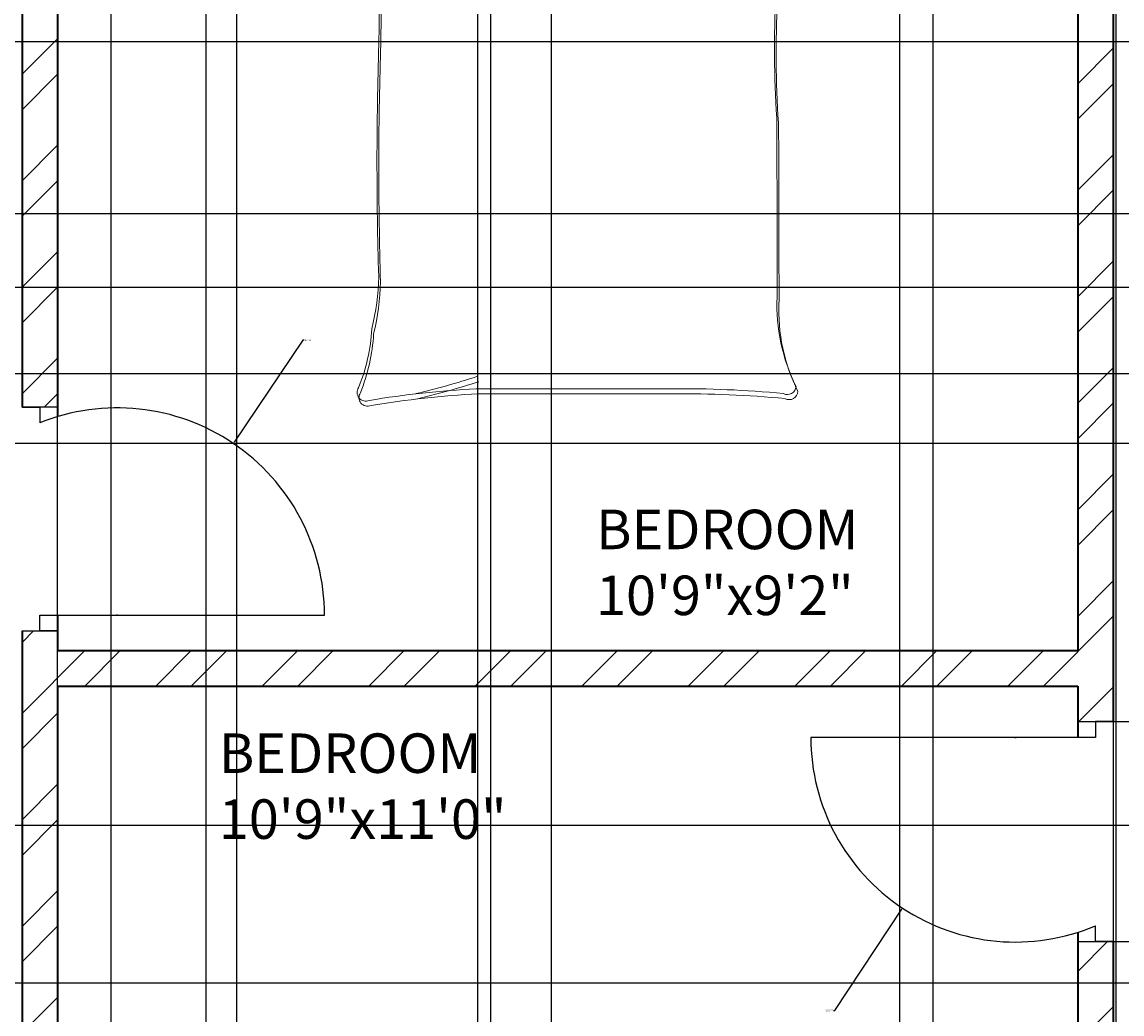
# Model space of a CAD drawing. Units: inches. Extents: x 2529 to 3014, y 1203 to 2262.
# Tile 11 of 13: x 2733 to 2872, y 2008 to 2133. Entities that reach past the tile are written whole.
import ezdxf

# ---------------------------------------------------------------- set-up
doc = ezdxf.new("R2010")
doc.units = ezdxf.units.IN
for name, color, linetype, lineweight in [('A-ANNO-DIMS', 2, 'Continuous', 18), ('A-AREA-IDEN', 7, 'Continuous', 18), ('A-DOOR', 21, 'Continuous', 25), ('A-FURN', 8, 'Continuous', 18), ('A-WALL', 7, 'Continuous', 35), ('A-WALL-PATT', 143, 'Continuous', 13)]:
    doc.layers.add(name, color=color, linetype=linetype, lineweight=lineweight)
doc.styles.get("Standard").update_dxf_attribs({"font": 'arial.ttf'})
doc.dimstyles.get("Standard").update_dxf_attribs({"dimtxt": 0.18, "dimasz": 0.18, "dimexe": 0.18, "dimexo": 0.0625, "dimgap": 0.09, "dimtad": 0, "dimtih": 1, "dimtoh": 1, "dimdec": 4, "dimzin": 0, "dimdsep": 46, "dimtxsty": 'Standard', "dimcen": 0.09, "dimadec": 0, "dimazin": 0, "dimtfac": 1, "dimtdec": 4, "dimtofl": 0, "dimtmove": 0, "dimatfit": 3, "dimfxl": 1, "dimtolj": 1, "dimtzin": 0, "dimarcsym": 0})

# ---------------------------------------------------------------- blocks, each defined once
blk = doc.blocks.new('BED-DOUBLE')
for p, q in [((3.48, 63.33), (3.48, 81.44)), ((3.48, 63.33), (3.48, 81.44)), ((3.48, 81.44), (51.49, 81.44)), ((3.7, 62.69), (3.7, 80.8)), ((3.7, 62.69), (3.7, 80.8)), ((51.27, 81.44), (51.27, 54.83)), ((51.27, 81.44), (51.27, 54.83)), ((51.49, 81.44), (51.49, 80.8)), ((51.49, 80.8), (51.49, 54.19)), ((51.49, 80.8), (51.49, 54.19)), ((3.48, 79.91), (51.27, 79.91)), ((3.48, 79.91), (51.27, 79.91)), ((24.54, 78.99), (25.98, 79.57)), ((24.54, 78.99), (25.98, 79.57)), ((25.98, 79.57), (26.56, 74.22)), ((25.98, 79.57), (26.56, 74.22)), ((3.7, 79.27), (51.49, 79.27)), ((3.7, 79.27), (51.49, 79.27)), ((3.9, 78.11), (8.18, 78.43)), ((3.9, 78.11), (8.18, 78.43)), ((3.9, 78.13), (4.47, 74.95)), ((3.9, 78.13), (4.47, 74.95)), ((8.18, 78.43), (8.29, 78.42)), ((8.18, 78.43), (8.29, 78.42)), ((8.29, 78.42), (12.11, 78.13)), ((8.29, 78.42), (12.11, 78.13)), ((12.11, 78.13), (17.6, 77.12)), ((12.11, 78.13), (17.6, 77.12)), ((14.86, 77.69), (16.88, 78.42)), ((14.86, 77.69), (16.88, 78.42)), ((16.88, 78.42), (19.77, 79.14)), ((16.88, 78.42), (19.77, 79.14)), ((17.11, 77.78), (20, 78.5)), ((17.11, 77.78), (20, 78.5)), ((19.77, 79.14), (20.09, 79.14)), ((19.77, 79.14), (20.09, 79.14)), ((20, 78.5), (20.32, 78.5)), ((20, 78.5), (20.32, 78.5)), ((20.09, 79.14), (24.54, 78.99)), ((20.09, 79.14), (24.54, 78.99)), ((20.32, 78.5), (24.77, 78.36)), ((20.32, 78.5), (24.77, 78.36)), ((24.77, 78.36), (26.21, 78.93)), ((24.77, 78.36), (26.21, 78.93)), ((26.21, 78.93), (26.79, 73.58)), ((26.21, 78.93), (26.79, 73.58)), ((27.98, 78.95), (27.73, 73.58)), ((27.98, 78.95), (27.73, 73.58)), ((28.21, 78.31), (27.96, 72.94)), ((28.21, 78.31), (27.96, 72.94)), ((29.46, 78.46), (27.98, 78.95)), ((29.46, 78.46), (27.98, 78.95)), ((29.68, 77.83), (28.21, 78.31)), ((29.68, 77.83), (28.21, 78.31)), ((33.88, 78.89), (29.46, 78.46)), ((33.88, 78.89), (29.46, 78.46)), ((34.11, 78.25), (29.68, 77.83)), ((34.11, 78.25), (29.68, 77.83)), ((34.21, 78.91), (33.88, 78.89)), ((34.21, 78.91), (33.88, 78.89)), ((34.43, 78.27), (34.11, 78.25)), ((34.43, 78.27), (34.11, 78.25)), ((37.14, 78.37), (34.21, 78.91)), ((37.14, 78.37), (34.21, 78.91)), ((37.36, 77.73), (34.43, 78.27)), ((37.36, 77.73), (34.43, 78.27)), ((41.91, 78.37), (36.5, 77.02)), ((41.91, 78.37), (36.5, 77.02)), ((39.2, 77.77), (37.14, 78.37)), ((39.2, 77.77), (37.14, 78.37)), ((45.71, 78.9), (41.91, 78.37)), ((45.71, 78.9), (41.91, 78.37)), ((45.94, 78.26), (42.14, 77.73)), ((45.94, 78.26), (42.14, 77.73)), ((50.11, 78.89), (44.71, 78.98)), ((44.71, 78.98), (45.71, 78.9)), ((50.11, 78.89), (44.71, 78.98)), ((44.71, 78.98), (45.71, 78.9)), ((50.34, 78.25), (44.94, 78.34)), ((44.94, 78.34), (45.94, 78.26)), ((50.34, 78.25), (44.94, 78.34)), ((44.94, 78.34), (45.94, 78.26)), ((50.11, 78.89), (49.73, 75.68)), ((50.11, 78.89), (49.73, 75.68)), ((50.34, 78.25), (49.96, 75.04)), ((50.34, 78.25), (49.96, 75.04)), ((4.12, 77.49), (4.7, 74.31)), ((4.12, 77.49), (4.7, 74.31)), ((4.13, 77.47), (8.41, 77.8)), ((4.13, 77.47), (8.41, 77.8)), ((8.41, 77.8), (8.51, 77.78)), ((8.41, 77.8), (8.51, 77.78)), ((8.51, 77.78), (12.34, 77.49)), ((8.51, 77.78), (12.34, 77.49)), ((12.34, 77.49), (17.83, 76.48)), ((12.34, 77.49), (17.83, 76.48)), ((15.08, 77.05), (17.11, 77.78)), ((15.08, 77.05), (17.11, 77.78)), ((42.14, 77.73), (36.72, 76.38)), ((42.14, 77.73), (36.72, 76.38)), ((39.43, 77.13), (37.36, 77.73)), ((39.43, 77.13), (37.36, 77.73)), ((5.05, 72.49), (6.06, 75.24)), ((5.05, 72.49), (6.06, 75.24)), ((49.31, 73.19), (48.13, 75.87)), ((49.31, 73.19), (48.13, 75.87)), ((49.54, 72.55), (48.36, 75.23)), ((49.54, 72.55), (48.36, 75.23)), ((49.73, 75.68), (50.33, 73.11)), ((49.73, 75.68), (50.33, 73.11)), ((4.47, 74.95), (4.04, 72.34)), ((4.47, 74.95), (4.04, 72.34)), ((4.7, 74.31), (4.27, 71.7)), ((4.7, 74.31), (4.27, 71.7)), ((5.28, 71.85), (6.29, 74.6)), ((5.28, 71.85), (6.29, 74.6)), ((26.56, 74.22), (27.14, 71.04)), ((26.56, 74.22), (27.14, 71.04)), ((49.96, 75.04), (50.56, 72.47)), ((49.96, 75.04), (50.56, 72.47)), ((4.04, 72.34), (4.62, 71.33)), ((4.04, 72.34), (4.62, 71.33)), ((4.47, 68.87), (5.05, 72.49)), ((4.47, 68.87), (5.05, 72.49)), ((26.79, 73.58), (27.37, 70.4)), ((26.79, 73.58), (27.37, 70.4)), ((27.73, 73.58), (27.36, 70.37)), ((27.73, 73.58), (27.36, 70.37)), ((27.96, 72.94), (27.58, 69.73)), ((27.96, 72.94), (27.58, 69.73)), ((50.11, 69.61), (49.31, 73.19)), ((50.11, 69.61), (49.31, 73.19)), ((50.34, 68.98), (49.54, 72.55)), ((50.34, 68.98), (49.54, 72.55)), ((50.33, 73.11), (49.81, 72.06)), ((50.33, 73.11), (49.82, 72.06)), ((50.56, 72.47), (50.04, 71.42)), ((50.56, 72.47), (50.04, 71.42)), ((4.27, 71.7), (4.85, 70.69)), ((4.27, 71.7), (4.85, 70.69)), ((4.7, 68.23), (5.28, 71.85)), ((4.7, 68.23), (5.28, 71.85)), ((27.14, 71.04), (27.14, 69.74)), ((27.14, 71.04), (27.14, 69.74)), ((27.14, 69.74), (26.56, 67.86)), ((27.14, 69.74), (26.56, 67.86)), ((27.36, 70.37), (27.44, 69.07)), ((27.36, 70.37), (27.44, 69.07)), ((27.37, 70.4), (27.37, 69.1)), ((27.37, 70.4), (27.37, 69.1)), ((27.58, 69.73), (27.67, 68.43)), ((27.58, 69.73), (27.66, 68.43)), ((49.92, 68.01), (50.11, 69.61)), ((49.92, 68.01), (50.11, 69.61)), ((4.76, 67.28), (4.47, 68.87)), ((4.76, 67.28), (4.47, 68.87)), ((4.99, 66.64), (4.7, 68.23)), ((4.99, 66.64), (4.7, 68.23)), ((27.37, 69.1), (26.79, 67.22)), ((27.37, 69.1), (26.79, 67.22)), ((27.44, 69.07), (28.13, 67.23)), ((27.44, 69.07), (28.13, 67.23)), ((27.66, 68.43), (28.36, 66.59)), ((27.67, 68.43), (28.36, 66.59)), ((50.15, 67.37), (50.34, 68.98)), ((50.15, 67.37), (50.34, 68.98)), ((4.18, 64.1), (4.76, 67.28)), ((4.18, 64.1), (4.76, 67.28)), ((26.56, 67.86), (26.56, 65.18)), ((26.56, 67.86), (26.56, 65.18)), ((26.79, 67.22), (26.79, 64.54)), ((26.79, 67.22), (26.79, 64.54)), ((28.13, 67.23), (28.3, 64.55)), ((28.13, 67.23), (28.3, 64.55)), ((50.7, 64.87), (49.92, 68.01)), ((50.7, 64.87), (49.92, 68.01)), ((50.93, 64.23), (50.15, 67.37)), ((50.93, 64.23), (50.15, 67.37)), ((4.41, 63.46), (4.99, 66.64)), ((4.41, 63.46), (4.99, 66.64)), ((6.38, 65.81), (10.41, 65.15)), ((6.38, 65.81), (10.41, 65.15)), ((24.1, 65.18), (20.96, 66.27)), ((24.1, 65.18), (20.96, 66.27)), ((24.33, 64.54), (21.19, 65.63)), ((24.33, 64.54), (21.19, 65.63)), ((28.36, 66.59), (28.53, 63.91)), ((28.36, 66.59), (28.53, 63.91)), ((30.75, 64.7), (33.82, 65.99)), ((30.75, 64.7), (33.82, 65.99)), ((32.56, 65.81), (36.6, 65.15)), ((32.56, 65.81), (36.6, 65.15)), ((9.28, 64.83), (4.18, 64.1)), ((9.28, 64.83), (4.18, 64.1)), ((9.51, 64.19), (4.41, 63.46)), ((9.51, 64.19), (4.41, 63.46)), ((6.61, 65.18), (10.64, 64.51)), ((6.61, 65.18), (10.64, 64.51)), ((10.41, 65.15), (9.28, 64.83)), ((10.41, 65.15), (9.28, 64.83)), ((10.64, 64.51), (9.51, 64.19)), ((10.64, 64.51), (9.51, 64.19)), ((10.41, 65.15), (17.42, 64.72)), ((10.41, 65.15), (17.42, 64.72)), ((10.64, 64.51), (17.65, 64.08)), ((10.64, 64.51), (17.65, 64.08)), ((17.42, 64.72), (19.38, 65.27)), ((17.42, 64.72), (19.38, 65.27)), ((17.65, 64.08), (19.61, 64.64)), ((17.65, 64.08), (19.61, 64.64)), ((19.38, 65.27), (24.52, 64.87)), ((19.38, 65.27), (24.52, 64.87)), ((19.61, 64.64), (24.74, 64.23)), ((19.61, 64.64), (24.74, 64.23)), ((26.56, 65.18), (24.1, 65.18)), ((26.56, 65.18), (24.1, 65.18)), ((26.79, 64.54), (24.33, 64.54)), ((26.79, 64.54), (24.33, 64.54)), ((28.3, 64.55), (30.75, 64.7)), ((28.3, 64.55), (30.75, 64.7)), ((28.53, 63.91), (30.98, 64.06)), ((28.53, 63.91), (30.98, 64.06)), ((30.26, 64.06), (34.45, 57.57)), ((30.26, 64.06), (34.45, 57.57)), ((30.98, 64.06), (34.05, 65.35)), ((30.98, 64.06), (34.05, 65.35)), ((40.64, 61.13), (32.31, 64.06)), ((40.64, 61.13), (32.31, 64.06)), ((32.79, 65.18), (36.83, 64.51)), ((32.79, 65.18), (36.82, 64.51)), ((36.6, 65.15), (43.61, 64.72)), ((36.6, 65.15), (43.61, 64.72)), ((36.82, 64.51), (43.83, 64.08)), ((36.83, 64.51), (43.84, 64.08)), ((43.61, 64.72), (45.57, 65.27)), ((43.61, 64.72), (45.57, 65.27)), ((43.83, 64.08), (45.8, 64.64)), ((43.84, 64.08), (45.8, 64.64)), ((45.57, 65.27), (50.7, 64.87)), ((45.57, 65.27), (50.7, 64.87)), ((45.8, 64.64), (50.93, 64.23)), ((45.8, 64.64), (50.93, 64.23)), ((30.49, 63.42), (34.68, 56.93)), ((30.49, 63.42), (34.68, 56.93)), ((40.87, 60.49), (32.53, 63.42)), ((40.87, 60.49), (32.54, 63.42)), ((46.22, 59.11), (40.64, 61.13)), ((46.22, 59.11), (40.64, 61.13)), ((46.45, 58.48), (40.87, 60.49)), ((46.45, 58.48), (40.87, 60.49)), ((49.16, 56.95), (46.22, 59.11)), ((49.16, 56.95), (46.22, 59.11)), ((49.39, 56.31), (46.45, 58.48)), ((49.39, 56.31), (46.45, 58.48)), ((34.45, 57.57), (36.15, 53.08)), ((34.45, 57.57), (36.15, 53.08)), ((34.68, 56.93), (36.38, 52.44)), ((34.68, 56.93), (36.38, 52.44)), ((52.87, 53.7), (49.16, 56.95)), ((52.87, 53.7), (49.16, 56.95)), ((53.1, 53.06), (49.39, 56.31)), ((53.1, 53.06), (49.39, 56.31)), ((36.15, 53.08), (36.46, 51.07)), ((36.15, 53.08), (36.46, 51.07)), ((40.95, 52.61), (44.36, 53.08)), ((40.95, 52.61), (44.36, 53.08)), ((44.36, 53.08), (48.23, 53.39)), ((44.36, 53.08), (48.23, 53.39)), ((48.23, 53.39), (51.33, 53.08)), ((48.23, 53.39), (51.33, 53.08)), ((51.33, 53.08), (52.87, 53.7)), ((51.33, 53.08), (52.87, 53.7)), ((51.56, 52.44), (53.1, 53.06)), ((51.56, 52.44), (53.1, 53.06)), ((52.95, 51.95), (52.87, 53.7, 3.87)), ((52.95, 51.95), (52.87, 53.7, 3.87)), ((53.18, 51.31), (53.1, 53.06, 3.87)), ((53.18, 51.31), (53.1, 53.06, 3.87)), ((36.38, 52.44), (36.69, 50.43)), ((36.38, 52.44), (36.69, 50.43)), ((36.46, 51.07), (38.94, 51.69)), ((36.46, 51.07), (38.94, 51.69)), ((38.94, 51.69), (40.95, 52.61)), ((38.94, 51.69), (40.95, 52.61)), ((39.17, 51.05), (41.18, 51.97)), ((39.17, 51.05), (41.18, 51.97)), ((41.18, 51.97), (44.59, 52.44)), ((41.18, 51.97), (44.59, 52.44)), ((44.59, 52.44), (48.46, 52.75)), ((44.59, 52.44), (48.46, 52.75)), ((48.46, 52.75), (51.56, 52.44)), ((48.46, 52.75), (51.56, 52.44)), ((36.69, 50.43), (39.17, 51.05)), ((36.69, 50.43), (39.17, 51.05)), ((15.06, 2.2), (39.68, 2.2)), ((15.06, 2.2), (39.68, 2.2)), ((15.29, 1.56), (39.91, 1.56)), ((15.29, 1.56), (39.91, 1.56))]:
    blk.add_line(p, q)
for centre, radius, start, end in [((21.36, -100.61), 164.97, 86.0865, 96.7821), ((21.36, -100.61), 164.97, 86.0865, 96.7821), ((85.16, 61.35), 83.31, 178.7218, 185.604), ((85.16, 61.35), 83.31, 178.7218, 185.604), ((21.59, -101.25), 164.97, 86.0865, 96.7821), ((21.59, -101.25), 164.97, 86.0865, 96.7821), ((85.39, 60.71), 83.31, 178.7218, 185.604), ((85.39, 60.71), 83.31, 178.7218, 185.604), ((17.76, -74.87), 129.02, 81.7845, 96.9006), ((17.76, -74.87), 129.02, 81.7845, 96.9006), ((17.98, -75.51), 129.02, 81.7845, 96.9006), ((17.98, -75.51), 129.02, 81.7845, 96.9006), ((-167.31, 50.27), 170.11, 358.4762, 1.0082), ((-167.31, 50.27), 170.11, 358.4762, 1.0082), ((-167.08, 49.63), 170.11, 358.4762, 1.0082), ((-167.08, 49.63), 170.11, 358.4762, 1.0082), ((31.15, 79.96), 29.65, 280.6617, 289.8806), ((31.15, 79.96), 29.65, 280.6617, 289.8806), ((43.74, 46.38), 6.22, 78.6608, 113.7384), ((43.74, 46.38), 6.22, 78.6608, 113.7384), ((43.97, 45.74), 6.22, 78.6608, 113.7384), ((43.97, 45.74), 6.22, 78.6608, 113.7384), ((51.33, 88.1), 36.18, 259.8763, 272.5657), ((51.33, 88.1), 36.18, 259.8763, 272.5657), ((51.56, 87.46), 36.18, 259.8763, 272.5657), ((51.56, 87.46), 36.18, 259.8763, 272.5657), ((182.27, 45.13), 129.5, 176.9791, 183.8365), ((182.27, 45.13), 129.5, 176.9791, 183.8365), ((36.64, 51), 0.185, 160.2464, 271.1377), ((36.64, 51), 0.185, 160.2464, 271.1377), ((36.87, 50.36), 0.185, 160.2464, 271.1377), ((36.86, 50.36), 0.185, 160.2464, 271.1377), ((31.38, 79.32), 29.65, 280.6617, 289.8806), ((31.38, 79.32), 29.65, 280.6617, 289.8806), ((182.49, 44.49), 129.5, 176.9791, 183.8365), ((182.49, 44.49), 129.5, 176.9791, 183.8365), ((484.82, 30.83), 482.31, 178.2277, 181.7185), ((484.82, 30.83), 482.31, 178.2277, 181.7185), ((485.05, 30.19), 482.31, 178.2277, 181.7185), ((485.05, 30.19), 482.31, 178.2277, 181.7185), ((-4508.74, 13.62), 4561.86, 0.00217, 0.28689), ((-4508.74, 13.62), 4561.86, 0.00217, 0.28689), ((-4508.51, 12.98), 4561.86, 0.00217, 0.28689), ((-4508.51, 12.98), 4561.86, 0.00217, 0.28689), ((-26.9, 16.93), 29.63, 346.0648, 358.9113), ((-26.9, 16.93), 29.63, 346.0648, 358.9113), ((-26.67, 16.29), 29.63, 346.0648, 358.9113), ((-26.67, 16.29), 29.63, 346.0648, 358.9113), ((76.16, 12.78), 23.07, 177.4714, 206.4681), ((76.16, 12.78), 23.07, 177.4714, 206.4681), ((76.39, 12.14), 23.07, 177.4714, 206.4681), ((76.39, 12.14), 23.07, 177.4714, 206.4681), ((-21.66, 11.17), 23.56, 337.9751, 356.652), ((-21.66, 11.17), 23.56, 337.9751, 356.652), ((-21.43, 10.53), 23.56, 337.9751, 356.652), ((-21.43, 10.53), 23.56, 337.9751, 356.652), ((-17.22, 105.16), 106.46, 283.3832, 287.7053), ((-17.22, 105.16), 106.46, 283.3832, 287.7053), ((-16.99, 104.52), 106.46, 283.3832, 287.7053), ((-16.99, 104.52), 106.46, 283.3832, 287.7053), ((1.09, 1.73), 1.09, 146.1736, 293.4781), ((1.09, 1.73), 1.09, 146.1736, 293.4781), ((1.32, 1.09), 1.09, 146.1736, 293.4781), ((1.32, 1.09), 1.09, 146.1736, 293.4781), ((21.43, -119.39), 121.76, 92.9958, 99.4091), ((21.43, -119.39), 121.76, 92.9958, 99.4091), ((21.66, -120.03), 121.76, 92.9958, 99.4091), ((21.66, -120.03), 121.76, 92.9958, 99.4091), ((41.15, -130.83), 133.04, 84.4998, 90.6351), ((41.15, -130.83), 133.04, 84.4998, 90.6351), ((41.38, -131.47), 133.04, 84.4998, 90.6351), ((41.38, -131.47), 133.04, 84.4998, 90.6351), ((54.41, 2.57), 1.1, 242.6588, 356.02), ((54.41, 2.57), 1.1, 242.6588, 356.02), ((54.64, 1.93), 1.1, 242.6588, 356.02), ((54.64, 1.93), 1.1, 242.6588, 356.02)]:
    blk.add_arc(centre, radius, start, end)
blk = doc.blocks.new('*D36')
at = {"layer": 'A-ANNO-DIMS', "color": 0, "lineweight": -2, "transparency": 16777216}
for p, q in [((2737.56, 1582.57), (2737.56, 2243.11)), ((2737.74, 2242.93), (2746.49, 2242.93)), ((2756.15, 2242.93), (2747.4, 2242.93)), ((2756.33, 1582.57), (2756.33, 2243.11))]:
    blk.add_line(p, q, dxfattribs=at)
at = {"layer": 'A-ANNO-DIMS', "color": 0, "transparency": 16777216}
for points in [[(2737.74, 2242.96), (2737.74, 2242.9), (2737.56, 2242.93)], [(2756.15, 2242.96), (2756.15, 2242.9), (2756.33, 2242.93)]]:
    blk.add_solid(points, dxfattribs=at)
at = {"layer": 'Defpoints', "color": 0, "transparency": 16777216}
for p in [(2756.33, 2242.93), (2737.56, 1582.5), (2756.33, 1582.5)]:
    blk.add_point(p, dxfattribs=at)
at = {"layer": 'A-ANNO-DIMS', "color": 0, "transparency": 16777216, "insert": (2746.94, 2242.93), "char_height": 0.18, "attachment_point": 5}
blk.add_mtext('\\A1;18.778', dxfattribs=at)
blk = doc.blocks.new('*D37')
at = {"layer": 'A-ANNO-DIMS', "color": 0, "lineweight": -2, "transparency": 16777216}
for p, q in [((2756.33, 1582.57), (2756.33, 2243.11)), ((2756.51, 2242.93), (2774.11, 2242.93)), ((2792.15, 2242.93), (2774.55, 2242.93)), ((2792.33, 1582.57), (2792.33, 2243.11))]:
    blk.add_line(p, q, dxfattribs=at)
at = {"layer": 'A-ANNO-DIMS', "color": 0, "transparency": 16777216}
for points in [[(2756.51, 2242.96), (2756.51, 2242.9), (2756.33, 2242.93)], [(2792.15, 2242.96), (2792.15, 2242.9), (2792.33, 2242.93)]]:
    blk.add_solid(points, dxfattribs=at)
at = {"layer": 'Defpoints', "color": 0, "transparency": 16777216}
for p in [(2792.33, 2242.93), (2756.33, 1582.5), (2792.33, 1582.5)]:
    blk.add_point(p, dxfattribs=at)
at = {"layer": 'A-ANNO-DIMS', "color": 0, "transparency": 16777216, "insert": (2774.33, 2242.93), "char_height": 0.18, "attachment_point": 5}
blk.add_mtext('\\A1;36', dxfattribs=at)
blk = doc.blocks.new('*D38')
at = {"layer": 'A-ANNO-DIMS', "color": 0, "lineweight": -2, "transparency": 16777216}
for p, q in [((2844.06, 1582.57), (2844.06, 2243.11)), ((2844.24, 2242.93), (2857.35, 2242.93)), ((2871.26, 2242.93), (2858.14, 2242.93)), ((2871.44, 1582.57), (2871.44, 2243.11))]:
    blk.add_line(p, q, dxfattribs=at)
at = {"layer": 'A-ANNO-DIMS', "color": 0, "transparency": 16777216}
for points in [[(2844.24, 2242.96), (2844.24, 2242.9), (2844.06, 2242.93)], [(2871.26, 2242.96), (2871.26, 2242.9), (2871.44, 2242.93)]]:
    blk.add_solid(points, dxfattribs=at)
at = {"layer": 'Defpoints', "color": 0, "transparency": 16777216}
for p in [(2871.44, 2242.93), (2844.06, 1582.5), (2871.44, 1582.5)]:
    blk.add_point(p, dxfattribs=at)
at = {"layer": 'A-ANNO-DIMS', "color": 0, "transparency": 16777216, "insert": (2857.75, 2242.93), "char_height": 0.18, "attachment_point": 5}
blk.add_mtext('\\A1;27.39', dxfattribs=at)
blk = doc.blocks.new('*D39')
at = {"layer": 'A-ANNO-DIMS', "color": 0, "lineweight": -2, "transparency": 16777216}
for p, q in [((2848.27, 1734.07), (2848.27, 2243.11)), ((2848.45, 2242.93), (2864.3, 2242.93)), ((2881.08, 2242.93), (2865.23, 2242.93)), ((2881.26, 1734.07), (2881.26, 2243.11))]:
    blk.add_line(p, q, dxfattribs=at)
at = {"layer": 'A-ANNO-DIMS', "color": 0, "transparency": 16777216}
for points in [[(2848.45, 2242.96), (2848.45, 2242.9), (2848.27, 2242.93)], [(2881.08, 2242.96), (2881.08, 2242.9), (2881.26, 2242.93)]]:
    blk.add_solid(points, dxfattribs=at)
at = {"layer": 'Defpoints', "color": 0, "transparency": 16777216}
for p in [(2881.26, 2242.93), (2848.27, 1734), (2881.26, 1734)]:
    blk.add_point(p, dxfattribs=at)
at = {"layer": 'A-ANNO-DIMS', "color": 0, "transparency": 16777216, "insert": (2864.76, 2242.93), "char_height": 0.18, "attachment_point": 5}
blk.add_mtext('\\A1;32.994', dxfattribs=at)
blk = doc.blocks.new('*D40')
at = {"layer": 'A-ANNO-DIMS', "color": 0, "lineweight": -2, "transparency": 16777216}
for p, q in [((2744.32, 1738.57), (2744.32, 2243.11)), ((2744.5, 2242.93), (2771.84, 2242.93)), ((2799.84, 2242.93), (2772.49, 2242.93)), ((2800.02, 1738.57), (2800.02, 2243.11))]:
    blk.add_line(p, q, dxfattribs=at)
at = {"layer": 'A-ANNO-DIMS', "color": 0, "transparency": 16777216}
for points in [[(2744.5, 2242.96), (2744.5, 2242.9), (2744.32, 2242.93)], [(2799.84, 2242.96), (2799.84, 2242.9), (2800.02, 2242.93)]]:
    blk.add_solid(points, dxfattribs=at)
at = {"layer": 'Defpoints', "color": 0, "transparency": 16777216}
for p in [(2800.02, 2242.93), (2744.32, 1738.5), (2800.02, 1738.5)]:
    blk.add_point(p, dxfattribs=at)
at = {"layer": 'A-ANNO-DIMS', "color": 0, "transparency": 16777216, "insert": (2772.17, 2242.93), "char_height": 0.18, "attachment_point": 5}
blk.add_mtext('\\A1;55.7', dxfattribs=at)
blk = doc.blocks.new('*D47')
at = {"layer": 'A-ANNO-DIMS', "color": 0, "lineweight": -2, "transparency": 16777216}
for p, q in [((2622.12, 2131.02), (3007.66, 2131.02)), ((3007.48, 2130.84), (3007.48, 2120.34)), ((3007.48, 2109.48), (3007.48, 2119.98)), ((2622.12, 2109.3), (3007.66, 2109.3))]:
    blk.add_line(p, q, dxfattribs=at)
at = {"layer": 'A-ANNO-DIMS', "color": 0, "transparency": 16777216}
for points in [[(3007.45, 2130.84), (3007.51, 2130.84), (3007.48, 2131.02)], [(3007.45, 2109.48), (3007.51, 2109.48), (3007.48, 2109.3)]]:
    blk.add_solid(points, dxfattribs=at)
at = {"layer": 'Defpoints', "color": 0, "transparency": 16777216}
for p in [(2622.06, 2131.02), (3007.48, 2131.02), (2622.06, 2109.3)]:
    blk.add_point(p, dxfattribs=at)
at = {"layer": 'A-ANNO-DIMS', "color": 0, "transparency": 16777216, "insert": (3007.48, 2120.16), "char_height": 0.18, "attachment_point": 5}
blk.add_mtext('\\A1;21.72', dxfattribs=at)
blk = doc.blocks.new('*D48')
at = {"layer": 'A-ANNO-DIMS', "color": 0, "lineweight": -2, "transparency": 16777216}
for p, q in [((2686.62, 2099.98), (3007.66, 2099.98)), ((3007.48, 2099.8), (3007.48, 2090.29)), ((3007.48, 2080.41), (3007.48, 2089.93)), ((2686.62, 2080.23), (3007.66, 2080.23))]:
    blk.add_line(p, q, dxfattribs=at)
at = {"layer": 'A-ANNO-DIMS', "color": 0, "transparency": 16777216}
for points in [[(3007.45, 2099.8), (3007.51, 2099.8), (3007.48, 2099.98)], [(3007.45, 2080.41), (3007.51, 2080.41), (3007.48, 2080.23)]]:
    blk.add_solid(points, dxfattribs=at)
at = {"layer": 'Defpoints', "color": 0, "transparency": 16777216}
for p in [(2686.56, 2099.98), (3007.48, 2099.98), (2686.56, 2080.23)]:
    blk.add_point(p, dxfattribs=at)
at = {"layer": 'A-ANNO-DIMS', "color": 0, "transparency": 16777216, "insert": (3007.48, 2090.11), "char_height": 0.18, "attachment_point": 5}
blk.add_mtext('\\A1;19.75', dxfattribs=at)
blk = doc.blocks.new('*D50')
at = {"layer": 'A-ANNO-DIMS', "color": 0, "lineweight": -2, "transparency": 16777216}
for p, q in [((2866.62, 2045.02), (3007.66, 2045.02)), ((3007.48, 2044.84), (3007.48, 2031.3)), ((3007.48, 2017.39), (3007.48, 2030.93)), ((2866.62, 2017.21), (3007.66, 2017.21))]:
    blk.add_line(p, q, dxfattribs=at)
at = {"layer": 'A-ANNO-DIMS', "color": 0, "transparency": 16777216}
for points in [[(3007.45, 2044.84), (3007.51, 2044.84), (3007.48, 2045.02)], [(3007.45, 2017.39), (3007.51, 2017.39), (3007.48, 2017.21)]]:
    blk.add_solid(points, dxfattribs=at)
at = {"layer": 'Defpoints', "color": 0, "transparency": 16777216}
for p in [(2866.56, 2045.02), (3007.48, 2045.02), (2866.56, 2017.21)]:
    blk.add_point(p, dxfattribs=at)
at = {"layer": 'A-ANNO-DIMS', "color": 0, "transparency": 16777216, "insert": (3007.48, 2031.12), "char_height": 0.18, "attachment_point": 5}
blk.add_mtext('\\A1;27.814', dxfattribs=at)
blk = doc.blocks.new('*D57')
at = {"layer": 'A-ANNO-DIMS', "color": 0, "lineweight": -2, "transparency": 16777216}
for p, q in [((2871.06, 2198.44), (2871.06, 1483.77)), ((2893.92, 2198.44), (2893.92, 1483.77)), ((2871.24, 1483.95), (2882.02, 1483.95)), ((2893.74, 1483.95), (2882.95, 1483.95))]:
    blk.add_line(p, q, dxfattribs=at)
at = {"layer": 'A-ANNO-DIMS', "color": 0, "transparency": 16777216}
for points in [[(2871.24, 1483.98), (2871.24, 1483.92), (2871.06, 1483.95)], [(2893.74, 1483.98), (2893.74, 1483.92), (2893.92, 1483.95)]]:
    blk.add_solid(points, dxfattribs=at)
at = {"layer": 'Defpoints', "color": 0, "transparency": 16777216}
for p in [(2871.06, 2198.5), (2893.92, 2198.5), (2893.92, 1483.95)]:
    blk.add_point(p, dxfattribs=at)
at = {"layer": 'A-ANNO-DIMS', "color": 0, "transparency": 16777216, "insert": (2882.49, 1483.95), "char_height": 0.18, "attachment_point": 5}
blk.add_mtext('\\A1;22.866', dxfattribs=at)
blk = doc.blocks.new('*D58')
at = {"layer": 'A-ANNO-DIMS', "color": 0, "lineweight": -2, "transparency": 16777216}
for p, q in [((2918.49, 2089), (2541.45, 2089)), ((2541.63, 2088.82), (2541.63, 2060.62)), ((2541.63, 2032.05), (2541.63, 2060.26)), ((2918.49, 2031.87), (2541.45, 2031.87))]:
    blk.add_line(p, q, dxfattribs=at)
at = {"layer": 'A-ANNO-DIMS', "color": 0, "transparency": 16777216}
for points in [[(2541.6, 2088.82), (2541.66, 2088.82), (2541.63, 2089)], [(2541.6, 2032.05), (2541.66, 2032.05), (2541.63, 2031.87)]]:
    blk.add_solid(points, dxfattribs=at)
at = {"layer": 'Defpoints', "color": 0, "transparency": 16777216}
for p in [(2918.56, 2089), (2541.63, 2031.87), (2918.56, 2031.87)]:
    blk.add_point(p, dxfattribs=at)
at = {"layer": 'A-ANNO-DIMS', "color": 0, "transparency": 16777216, "insert": (2541.63, 2060.44), "char_height": 0.18, "attachment_point": 5}
blk.add_mtext('\\A1;57.13', dxfattribs=at)
blk = doc.blocks.new('*D59')
at = {"layer": 'A-ANNO-DIMS', "color": 0, "lineweight": -2, "transparency": 16777216}
for p, q in [((2918.49, 2031.87), (2541.45, 2031.87)), ((2541.63, 2031.69), (2541.63, 2022.09)), ((2541.63, 2012.12), (2541.63, 2021.73)), ((2918.49, 2011.94), (2541.45, 2011.94))]:
    blk.add_line(p, q, dxfattribs=at)
at = {"layer": 'A-ANNO-DIMS', "color": 0, "transparency": 16777216}
for points in [[(2541.6, 2031.69), (2541.66, 2031.69), (2541.63, 2031.87)], [(2541.6, 2012.12), (2541.66, 2012.12), (2541.63, 2011.94)]]:
    blk.add_solid(points, dxfattribs=at)
at = {"layer": 'Defpoints', "color": 0, "transparency": 16777216}
for p in [(2918.56, 2031.87), (2541.63, 2011.94), (2918.56, 2011.94)]:
    blk.add_point(p, dxfattribs=at)
at = {"layer": 'A-ANNO-DIMS', "color": 0, "transparency": 16777216, "insert": (2541.63, 2021.91), "char_height": 0.18, "attachment_point": 5}
blk.add_mtext('\\A1;19.933', dxfattribs=at)
blk = doc.blocks.new('*D78')
at = {"layer": 'A-ANNO-DIMS', "color": 0, "lineweight": -2, "transparency": 16777216}
for p, q in [((2760.22, 1599.16), (2760.22, 2243.11)), ((2760.4, 2242.93), (2775.15, 2242.93)), ((2790.54, 2242.93), (2775.8, 2242.93)), ((2790.72, 1599.16), (2790.72, 2243.11))]:
    blk.add_line(p, q, dxfattribs=at)
at = {"layer": 'A-ANNO-DIMS', "color": 0, "transparency": 16777216}
for points in [[(2760.4, 2242.96), (2760.4, 2242.9), (2760.22, 2242.93)], [(2790.54, 2242.96), (2790.54, 2242.9), (2790.72, 2242.93)]]:
    blk.add_solid(points, dxfattribs=at)
at = {"layer": 'Defpoints', "color": 0, "transparency": 16777216}
for p in [(2790.72, 2242.93), (2760.22, 1599.1), (2790.72, 1599.1)]:
    blk.add_point(p, dxfattribs=at)
at = {"layer": 'A-ANNO-DIMS', "color": 0, "transparency": 16777216, "insert": (2775.47, 2242.93), "char_height": 0.18, "attachment_point": 5}
blk.add_mtext('\\A1;30.5', dxfattribs=at)
blk = doc.blocks.new('*D85')
at = {"layer": 'A-ANNO-DIMS', "color": 0, "lineweight": -2, "transparency": 16777216}
for p, q in [((2768.57, 2093.24), (2759.87, 2080.36)), ((2768.75, 2093.24), (2768.57, 2093.24)), ((2745, 2058.49), (2745.18, 2058.49)), ((2745.09, 2058.4), (2745.09, 2058.58))]:
    blk.add_line(p, q, dxfattribs=at)
at = {"layer": 'A-ANNO-DIMS', "color": 0, "transparency": 16777216}
blk.add_solid([(2759.84, 2080.38), (2759.89, 2080.34), (2759.76, 2080.21)], dxfattribs=at)
at = {"layer": 'Defpoints', "color": 0, "transparency": 16777216}
for p in [(2759.76, 2080.21), (2745.09, 2058.49)]:
    blk.add_point(p, dxfattribs=at)
at = {"layer": 'A-ANNO-DIMS', "color": 0, "transparency": 16777216, "insert": (2769.21, 2093.24), "char_height": 0.18, "attachment_point": 5}
blk.add_mtext('\\A1;R26.21', dxfattribs=at)
blk = doc.blocks.new('*D86')
at = {"layer": 'A-ANNO-DIMS', "color": 0, "lineweight": -2, "transparency": 16777216}
for p, q in [((2858.59, 2043.02), (2858.77, 2043.02)), ((2858.68, 2042.93), (2858.68, 2043.11)), ((2835.84, 2008.49), (2844.31, 2021.29)), ((2835.66, 2008.49), (2835.84, 2008.49))]:
    blk.add_line(p, q, dxfattribs=at)
at = {"layer": 'A-ANNO-DIMS', "color": 0, "transparency": 16777216}
blk.add_solid([(2844.28, 2021.31), (2844.33, 2021.27), (2844.41, 2021.44)], dxfattribs=at)
at = {"layer": 'Defpoints', "color": 0, "transparency": 16777216}
for p in [(2858.68, 2043.02), (2844.41, 2021.44)]:
    blk.add_point(p, dxfattribs=at)
at = {"layer": 'A-ANNO-DIMS', "color": 0, "transparency": 16777216, "insert": (2835.11, 2008.49), "char_height": 0.18, "attachment_point": 5}
blk.add_mtext('\\A1;R25.877', dxfattribs=at)

msp = doc.modelspace()

# ---------------------------------------------------------------- hatches: boundary and pattern name
at = {"layer": 'A-WALL-PATT'}
h = msp.add_hatch(dxfattribs=at)
h.set_pattern_fill('ANSI32', color=256)
h.paths.add_polyline_path([(2686.5554, 2106.5032), (2622.0554, 2106.5032), (2622.0554, 2109.2964), (2617.4223, 2109.2964), (2613.0554, 2109.2964), (2613.0554, 2106.5032), (2577.0554, 2106.5032), (2577.0554, 2092.6918), (2586.0554, 2092.6918), (2586.0554, 2102.0032), (2682.0554, 2102.0032), (2682.0554, 2099.9833), (2686.5554, 2099.9833), (2686.5554, 2102.0032)])
h.paths.add_polyline_path([(2695.2249, 2054.0032), (2686.5554, 2054.0032), (2686.5554, 2080.2316), (2684.3054, 2080.2316), (2682.0554, 2080.2316), (2682.0554, 2054.0032), (2586.0554, 2054.0032), (2586.0554, 2068.6918), (2577.0554, 2068.6918), (2577.0554, 2019.1229), (2586.0554, 2019.1229), (2586.0554, 2049.5032), (2695.2249, 2049.5032)])
h.paths.add_polyline_path([(2737.5554, 2049.5032), (2866.5554, 2049.5032), (2866.5554, 2045.0233), (2871.0554, 2045.0233), (2871.0554, 2049.5032), (2871.0554, 2172.5032), (2866.5554, 2172.5032), (2829.1265, 2172.5032), (2829.1265, 2168.0032), (2866.5554, 2168.0032), (2866.5554, 2054.0032), (2737.5554, 2054.0032), (2737.5554, 2056.4892), (2735.3054, 2056.4892), (2733.0554, 2056.4892), (2733.0554, 2049.5032), (2733.0554, 1917.5032), (2733.0554, 1913.0032), (2871.0554, 1913.0032), (2871.0554, 1924.9149), (2868.8054, 1924.9149), (2866.5554, 1924.9149), (2866.5554, 1917.5032), (2737.5554, 1917.5032)], flags=17)
h.paths.add_polyline_path([(2972.0554, 2207.5032), (2613.0554, 2207.5032), (2613.0554, 2205.5032), (2613.0554, 2188.9366), (2622.0554, 2188.9366), (2622.0554, 2198.5032), (2733.0554, 2198.5032), (2733.0554, 2084.8053), (2735.3054, 2084.8053), (2737.5554, 2084.8053), (2737.5554, 2168.0032), (2769.1265, 2168.0032), (2769.1265, 2170.2532), (2769.1265, 2172.5032), (2737.5554, 2172.5032), (2737.5554, 2198.5032), (2963.0554, 2198.5032), (2963.0554, 2093.5032), (2912.0586, 2093.5032), (2912.0586, 2089.0032), (2918.5554, 2089.0032), (2918.5554, 2031.8749), (2923.0554, 2031.8749), (2923.0554, 2089.0032), (2963.0554, 2089.0032), (2963.0554, 2010.0032), (2923.0554, 2010.0032), (2923.0554, 2011.9417), (2918.5554, 2011.9417), (2918.5554, 2003.1338), (2923.0554, 2003.1338), (2923.0554, 2005.5032), (2963.0554, 2005.5032), (2963.0554, 1917.5032), (2963.0554, 1691.0776), (2972.0554, 1691.0776), (2972.0554, 1917.5032)])
h.paths.add_polyline_path([(2963.0554, 1945.5032), (2923.0554, 1945.5032), (2923.0554, 1983.0571), (2920.8054, 1983.0571), (2918.5554, 1983.0571), (2918.5554, 1941.0032), (2963.0554, 1941.0032)], flags=17)
h.paths.add_polyline_path([(2930.3679, 1788.7532), (2930.3679, 1791.0032), (2894.8637, 1791.0032), (2894.8637, 1786.5032), (2900.5554, 1786.5032), (2900.5554, 1784.6931), (2905.0554, 1784.6931), (2905.0554, 1786.5032), (2930.3679, 1786.5032)], flags=17)
h.paths.add_polyline_path([(2963.0554, 1791.0032), (2954.3679, 1791.0032), (2954.3679, 1786.5032), (2963.0554, 1786.5032)], flags=17)
h.paths.add_polyline_path([(2871.0554, 1853.0032), (2919.0554, 1853.0032), (2919.0554, 1847.0972), (2923.5554, 1847.0972), (2923.5554, 1853.0032), (2923.5554, 1857.5032), (2871.0554, 1857.5032), (2871.0554, 1871.7024), (2866.5554, 1871.7024), (2866.5554, 1791.0032), (2737.5554, 1791.0032), (2737.5554, 1806.6712), (2735.3054, 1806.6712), (2733.0554, 1806.6712), (2733.0554, 1791.0032), (2733.0554, 1786.5032), (2733.0554, 1780.6235), (2737.5554, 1780.6235), (2737.5554, 1786.5032), (2872.8745, 1786.5032), (2872.8745, 1788.7532), (2872.8745, 1791.0032), (2871.0554, 1791.0032)], flags=17)
h.paths.add_polyline_path([(2844.0554, 1734.0032), (2848.2652, 1734.0032), (2848.2652, 1738.5032), (2800.0167, 1738.5032), (2800.0167, 1734.0032), (2839.5554, 1734.0032), (2839.5554, 1582.5032), (2792.3334, 1582.5032), (2792.3334, 1573.5032), (2871.4433, 1573.5032), (2871.4433, 1578.0032), (2871.4433, 1582.5032), (2844.0554, 1582.5032)])
h.paths.add_polyline_path([(2972.0554, 1631.0776), (2963.0554, 1631.0776), (2963.0554, 1582.5032), (2931.4433, 1582.5032), (2931.4433, 1573.5032), (2972.0554, 1573.5032)])
h.paths.add_polyline_path([(2756.3334, 1582.5032), (2737.5554, 1582.5032), (2737.5554, 1734.0032), (2744.3201, 1734.0032), (2744.3201, 1738.5032), (2737.5554, 1738.5032), (2737.5554, 1746.0094), (2733.0554, 1746.0094), (2733.0554, 1738.5032), (2733.0554, 1612.5032), (2728.2475, 1612.5032), (2728.2475, 1603.5032), (2733.0554, 1603.5032), (2733.0554, 1582.5032), (2733.0554, 1573.5032), (2756.3334, 1573.5032), (2756.3334, 1578.0032)])
h.paths.add_polyline_path([(2695.7662, 1612.5032), (2658.4771, 1612.5032), (2658.4771, 1603.5032), (2695.7662, 1603.5032), (2695.7662, 1608.0032)])
h.paths.add_polyline_path([(2586.0554, 1686.9483), (2577.0554, 1686.9483), (2577.0554, 1603.5032), (2598.4771, 1603.5032), (2598.4771, 1608.0032), (2598.4771, 1612.5032), (2586.0554, 1612.5032)])
h.paths.add_polyline_path([(2683.2727, 1791.0032), (2586.0554, 1791.0032), (2586.0554, 1815.6736), (2581.5554, 1815.6736), (2577.0554, 1815.6736), (2577.0554, 1746.9483), (2586.0554, 1746.9483), (2586.0554, 1786.5032), (2683.2727, 1786.5032)])
h.paths.add_polyline_path([(2586.0554, 1959.1229), (2577.0554, 1959.1229), (2577.0554, 1875.6736), (2586.0554, 1875.6736), (2586.0554, 1913.0032), (2683.2727, 1913.0032), (2683.2727, 1917.5032), (2586.0554, 1917.5032)])
h = msp.add_hatch(dxfattribs=at)
h.set_pattern_fill('ANSI32', color=256)
h.paths.add_polyline_path([(2871.0554, 2017.2091), (2868.8054, 2017.2091), (2866.5554, 2017.2091), (2866.5554, 1984.9149), (2871.0554, 1984.9149)])
h.paths.add_polyline_path([(2755.9438, 2027.3569), (2794.7842, 2027.3569), (2794.7842, 2046.0142), (2755.9438, 2046.0142)], flags=9)

# ---------------------------------------------------------------- linework, layer by layer
at = {"layer": 'A-DOOR'}
for p, q in [((2737.5554, 2084.8053), (2733.0554, 2084.8053)), ((2733.0554, 2084.8053), (2735.3054, 2084.8053)), ((2735.3054, 2084.8053), (2735.3054, 2082.8053)), ((2735.3054, 2056.4892), (2735.3054, 2058.4892)), ((2735.3054, 2058.4892), (2771.3054, 2058.4892)), ((2733.0554, 2056.4892), (2737.5554, 2056.4892)), ((2737.5554, 2056.4892), (2735.3054, 2056.4892)), ((2866.5554, 2045.0233), (2871.0554, 2045.0233)), ((2871.0554, 2045.0233), (2868.8054, 2045.0233)), ((2868.8054, 2045.0233), (2868.8054, 2043.0233)), ((2868.8054, 2043.0233), (2832.8054, 2043.0233)), ((2868.8054, 2017.2091), (2868.8054, 2019.2091)), ((2866.5554, 2017.2091), (2871.0554, 2017.2091)), ((2871.0554, 2017.2091), (2868.8054, 2017.2091))]:
    msp.add_line(p, q, dxfattribs=at)
for centre, radius, start, end in [((2745.0932, 2058.4892), 26.2122, 0, 111.926004), ((2858.682, 2043.0233), 25.8766, 180, 293.030242)]:
    msp.add_arc(centre, radius, start, end, dxfattribs=at)
at = {"layer": 'A-WALL'}
for p, q in [((2733.0554, 2198.5032), (2733.0554, 2084.8053)), ((2871.0554, 2172.5032), (2871.0554, 2049.5032)), ((2737.5554, 2168.0032), (2737.5554, 2083.5941)), ((2866.5554, 2168.0032), (2866.5554, 2054.0032)), ((2871.0554, 2093.5032), (2871.0554, 2089.0032)), ((2737.5554, 2058.4892), (2737.5554, 2054.0032)), ((2733.0554, 2056.4892), (2733.0554, 2049.5032)), ((2737.5554, 2054.0032), (2866.5554, 2054.0032)), ((2733.0554, 2049.5032), (2733.0554, 1917.5032)), ((2737.5554, 2049.5032), (2737.5554, 1917.5032)), ((2737.5554, 2049.5032), (2866.5554, 2049.5032)), ((2866.5554, 2049.5032), (2866.5554, 2043.0233)), ((2871.0554, 2049.5032), (2871.0554, 2045.0233)), ((2866.5554, 2018.3735), (2866.5554, 1984.9149)), ((2871.0554, 2017.2091), (2871.0554, 1984.9149))]:
    msp.add_line(p, q, dxfattribs=at)

# ---------------------------------------------------------------- block references
at = {"layer": 'A-FURN'}
msp.add_blockref('BED-DOUBLE', (2775.436, 2084.91), dxfattribs=at)

# ---------------------------------------------------------------- texts
at = {"layer": 'A-AREA-IDEN', "char_height": 5, "attachment_point": 1}
for s, width, insert in [('BEDROOM\\P10\'9"x9\'2"', 137.257698, (2805.6516, 2071.8255)), ('BEDROOM\\P10\'9"x11\'0"', 137.938433, (2757.9544, 2043.5296))]:
    msp.add_mtext_dynamic_manual_height_columns(s, width=width, gutter_width=12.5, heights=[0], dxfattribs=dict(at, insert=insert))

# ---------------------------------------------------------------- dimensions: what is measured, and where the dimension line sits
at = {"layer": 'A-ANNO-DIMS'}
for base, p1, p2, override, picture, middle in [((2756.3334, 2242.9282), (2737.5554, 1582.5032), (2756.3334, 1582.5032), {"dimdec": 3, "dimlfac": 1, "dimrnd": 0, "dimzin": 0, "dimdsep": 46, "dimlunit": 2}, '*D36', (2746.9444, 2242.9282)), ((2800.0167, 2242.9282), (2744.3201, 1738.5032), (2800.0167, 1738.5032), {"dimdec": 1, "dimlfac": 1, "dimrnd": 0, "dimzin": 0, "dimdsep": 46, "dimlunit": 2}, '*D40', (2772.1684, 2242.9282)), ((2792.3334, 2242.9282), (2756.3334, 1582.5032), (2792.3334, 1582.5032), {"dimdec": 0, "dimlfac": 1, "dimrnd": 0, "dimzin": 0, "dimdsep": 46, "dimlunit": 2}, '*D37', (2774.3334, 2242.9282)), ((2790.721, 2242.9282), (2760.2227, 1599.0994), (2790.721, 1599.0994), {"dimdec": 1, "dimlfac": 1, "dimrnd": 0, "dimzin": 0, "dimdsep": 46, "dimlunit": 2}, '*D78', (2775.4718, 2242.9282)), ((2871.4433, 2242.9282), (2844.0554, 1582.5032), (2871.4433, 1582.5032), {"dimdec": 2, "dimlfac": 1, "dimrnd": 0, "dimzin": 0, "dimdsep": 46, "dimlunit": 2}, '*D38', (2857.7493, 2242.9282)), ((2881.259, 2242.9282), (2848.2652, 1734.0032), (2881.259, 1734.0032), {"dimdec": 3, "dimlfac": 1, "dimrnd": 0, "dimzin": 0, "dimdsep": 46, "dimlunit": 2}, '*D39', (2864.7621, 2242.9282)), ((2893.9216, 1483.9492), (2871.0554, 2198.5032), (2893.9216, 2198.5032), {"dimdec": 3, "dimlfac": 1, "dimrnd": 0, "dimzin": 0, "dimdsep": 46, "dimlunit": 2}, '*D57', (2882.4885, 1483.9492))]:
    dim = msp.add_linear_dim(base=base, p1=p1, p2=p2, dimstyle='Standard', override=override, dxfattribs=at)
    dim.commit()
    dim.dimension.update_dxf_attribs({"geometry": picture, "text_midpoint": middle})
for base, p1, p2, override, picture, middle in [((3007.4804, 2131.0168), (2622.0554, 2109.2964), (2622.0554, 2131.0168), {"dimdec": 2, "dimlfac": 1, "dimrnd": 0, "dimzin": 0, "dimdsep": 46, "dimlunit": 2}, '*D47', (3007.4804, 2120.1566)), ((3007.4804, 2099.9833), (2686.5554, 2080.2316), (2686.5554, 2099.9833), {"dimdec": 2, "dimlfac": 1, "dimrnd": 0, "dimzin": 0, "dimdsep": 46, "dimlunit": 2}, '*D48', (3007.4804, 2090.1074)), ((2541.6304, 2031.8749), (2918.5554, 2089.0032), (2918.5554, 2031.8749), {"dimdec": 2, "dimlfac": 1, "dimrnd": 0, "dimzin": 0, "dimdsep": 46, "dimlunit": 2}, '*D58', (2541.6304, 2060.4391)), ((3007.4804, 2045.0233), (2866.5554, 2017.2091), (2866.5554, 2045.0233), {"dimdec": 3, "dimlfac": 1, "dimrnd": 0, "dimzin": 0, "dimdsep": 46, "dimlunit": 2}, '*D50', (3007.4804, 2031.1162)), ((2541.6304, 2011.9417), (2918.5554, 2031.8749), (2918.5554, 2011.9417), {"dimdec": 3, "dimlfac": 1, "dimrnd": 0, "dimzin": 0, "dimdsep": 46, "dimlunit": 2}, '*D59', (2541.6304, 2021.9083))]:
    dim = msp.add_linear_dim(base=base, p1=p1, p2=p2, angle=90, dimstyle='Standard', override=override, dxfattribs=at)
    dim.commit()
    dim.dimension.update_dxf_attribs({"geometry": picture, "text_midpoint": middle})
for center, mpoint, override, picture, middle in [((2745.0932, 2058.4892), (2759.7648, 2080.2106), {"dimdec": 2, "dimlfac": 1, "dimrnd": 0, "dimzin": 0, "dimdsep": 46, "dimlunit": 2}, '*D85', (2769.2101, 2093.2435)), ((2858.682, 2043.0233), (2844.4053, 2021.4415), {"dimdec": 3, "dimlfac": 1, "dimrnd": 0, "dimzin": 0, "dimdsep": 46, "dimlunit": 2}, '*D86', (2835.1095, 2008.4923))]:
    dim = msp.add_radius_dim(center=center, mpoint=mpoint, dimstyle='Standard', override=override, dxfattribs=at)
    dim.commit()
    dim.dimension.update_dxf_attribs({"geometry": picture, "text_midpoint": middle, "dimtype": 164})

doc.saveas('drawing.dxf')
